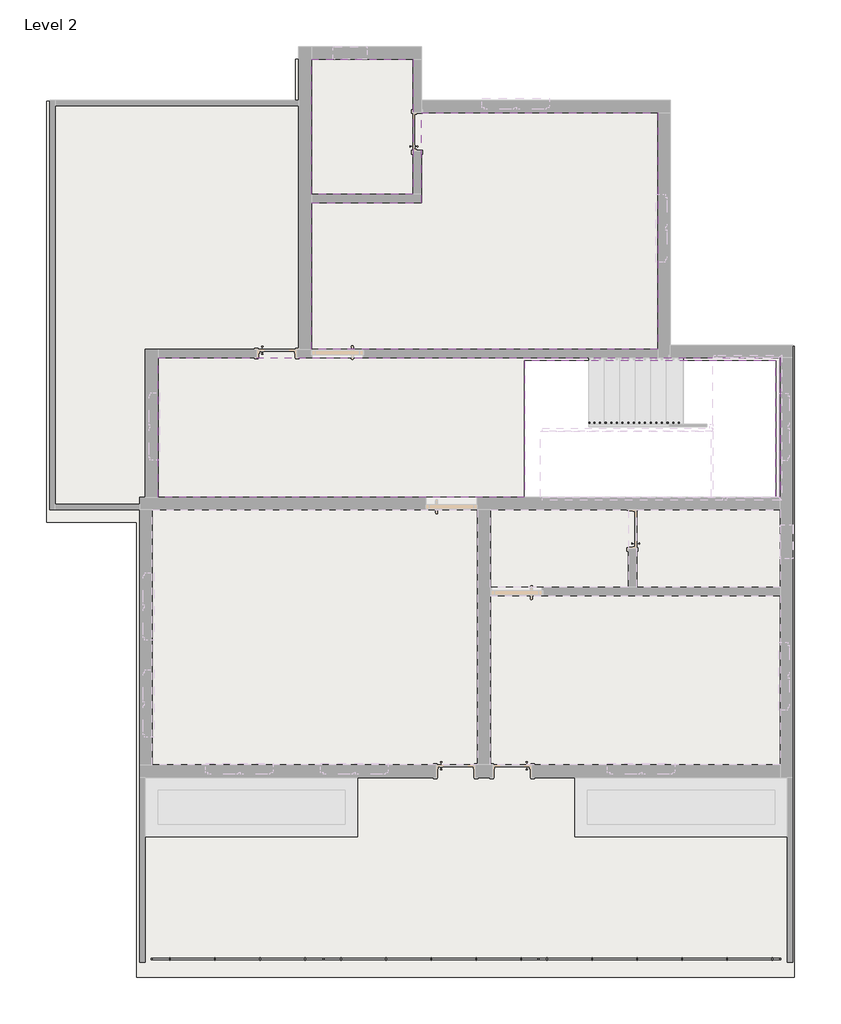
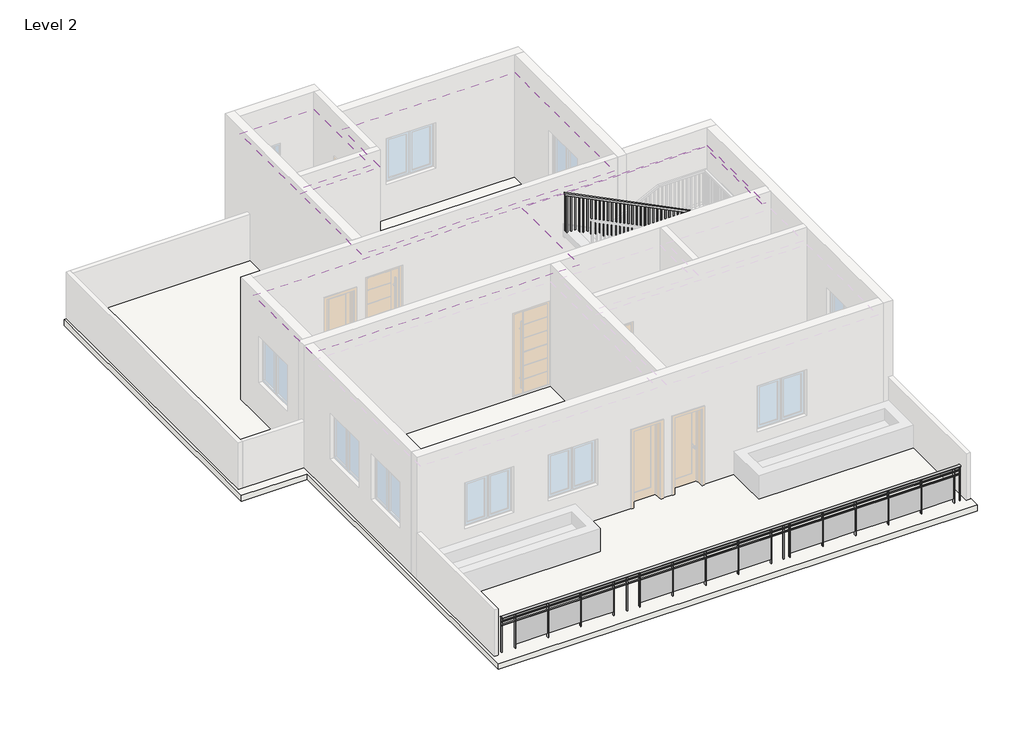
# One storey, part 2 of 3: 3 coverings, 2 railings, 1 slab.
"""IFC4 building model written with IfcOpenShell, lengths in millimetres."""

from ifc_helpers import new_model, si_unit, point, frame, origin, place, context, project, spatial, polyline, ellipse_curve, trimmed, outline, extrude, faceted_brep, element, save
from ifc_brep_helpers import plane_surface, extruded_surface, advanced_brep

model = new_model("IFC4")

# Units and contexts
model_context = context("Model", 3, world=origin())
ifc_project = project(units=[si_unit("LENGTHUNIT", "METRE", prefix="MILLI")], contexts=[model_context])

# Site, building, storey
site = spatial("IfcSite", under=ifc_project)
building = spatial("IfcBuilding", under=site)
storey = spatial("IfcBuildingStorey", under=building, Name="Level 2", Elevation=3200.4)

# Coverings
placement = place(None, origin())
element("IfcCovering", 1, ObjectType="2' x 4' ACT System", at=placement, inside=storey, context=model_context, shape_type="SweptSolid", body=[
    extrude(outline(polyline([(-10924.6183666, 3536.1503619), (-17173.0183666, 3536.1503619), (-17173.0183666, 6177.7503619), (-15191.8183666, 6177.7503619), (-15191.8183666, 7803.3503619), (-10924.6183666, 7803.3503619), (-10924.6183666, 3536.1503619)])), frame((0.0, 0.0, 6248.4), z_axis=(0.0, 0.0, 1.0), x_axis=(1.0, 0.0, 0.0)), (0.0, 0.0, 1.0), 57.15),
])
element("IfcCovering", 2, ObjectType="2' x 4' ACT System", at=placement, inside=storey, context=model_context, shape_type="SweptSolid", body=[
    extrude(outline(polyline([(-19941.6183666, 3383.7503619), (-10810.3183666, 3383.7503619), (-8714.8183666, 3383.7503619), (-8714.8183666, 869.1503619), (-8791.0183666, 869.1503619), (-8791.0183666, 3332.9503619), (-13326.4629678, 3332.9503619), (-13326.4629678, 869.1503619), (-19941.6183666, 869.1503619), (-19941.6183666, 3383.7503619)])), frame((0.0, 0.0, 6248.4), z_axis=(0.0, 0.0, 1.0), x_axis=(1.0, 0.0, 0.0)), (0.0, 0.0, 1.0), 57.15),
])
element("IfcCovering", 3, ObjectType="2' x 4' ACT System", at=placement, inside=storey, context=model_context, shape_type="SweptSolid", body=[
    extrude(outline(polyline([(-15344.2183666, 6330.1503619), (-17173.0183666, 6330.1503619), (-17173.0183666, 8768.5503619), (-15344.2183666, 8768.5503619), (-15344.2183666, 6330.1503619)])), frame((0.0, 0.0, 6248.4), z_axis=(0.0, 0.0, 1.0), x_axis=(1.0, 0.0, 0.0)), (0.0, 0.0, 1.0), 57.15),
])

# Railings
element("IfcRailing", 4, ObjectType="Glass Panel - Bottom Fill", at=placement, inside=storey, context=model_context, shape_type="SolidModel", body=[
    advanced_brep(
    [(-8708.4683666, -7493.7996381, 4419.6), (-8708.4683666, -7417.5996381, 4419.6), (-20062.2683666, -7493.7996381, 4419.6), (-20062.2683666, -7417.5996381, 4419.6)],
    [
        (0, 1, ellipse_curve(frame((-8708.4683666, -7455.6996381, 4419.6), z_axis=(1.0, 0.0, 0.0), x_axis=(0.0, 1.0, 0.0)), 38.1, 28.575)),
        (1, 0, ellipse_curve(frame((-8708.4683666, -7455.6996381, 4419.6), z_axis=(1.0, 0.0, 0.0), x_axis=(0.0, 1.0, 0.0)), 38.1, 28.575)),
        (2, 3, ellipse_curve(frame((-20062.2683666, -7455.6996381, 4419.6), z_axis=(-1.0, 0.0, 0.0), x_axis=(0.0, 1.0, 0.0)), 38.1, 28.575)),
        (3, 2, ellipse_curve(frame((-20062.2683666, -7455.6996381, 4419.6), z_axis=(-1.0, 0.0, 0.0), x_axis=(0.0, 1.0, 0.0)), 38.1, 28.575)),
        (0, 2),
        (3, 1),
    ],
    [
        plane_surface(frame((-8708.4683666, -7455.6996381, 4419.6), z_axis=(1.0, 0.0, 0.0), x_axis=(0.0, -1.0, 0.0))),
        plane_surface(frame((-20062.2683666, -7455.6996381, 4419.6), z_axis=(-1.0, 0.0, 0.0), x_axis=(0.0, -1.0, 0.0))),
        extruded_surface(trimmed(ellipse_curve(frame((-20062.2683666, -7455.6996381, 4419.6), z_axis=(1.0, 0.0, 0.0), x_axis=(0.0, 1.0, 0.0)), 38.1, 28.575), [point((-20062.2683666, -7493.7996381, 4419.6))], [point((-20062.2683666, -7417.5996381, 4419.6))], True, "CARTESIAN"), (11353.800000000001, 0.0, 0.0), 11353.800000000001),
        extruded_surface(trimmed(ellipse_curve(frame((-20062.2683666, -7455.6996381, 4419.6), z_axis=(1.0, 0.0, 0.0), x_axis=(0.0, 1.0, 0.0)), 38.1, 28.575), [point((-20062.2683666, -7417.5996381, 4419.6))], [point((-20062.2683666, -7493.7996381, 4419.6))], True, "CARTESIAN"), (11353.800000000001, 0.0, 0.0), 11353.800000000001),
    ],
    [
        (0, [[1, 2]]),
        (1, [[3, 4]]),
        (2, [[-1, 5, -4, 6]]),
        (3, [[-2, -6, -3, -5]]),
    ],
),
    extrude(outline(polyline([(-8708.4683666, -7442.9996381), (-8708.4683666, -7468.3996381), (-20062.2683666, -7468.3996381), (-20062.2683666, -7442.9996381), (-8708.4683666, -7442.9996381)])), frame((0.0, 0.0, 4305.3), z_axis=(0.0, 0.0, 1.0), x_axis=(1.0, 0.0, 0.0)), (0.0, 0.0, 1.0), 25.4),
    extrude(outline(polyline([(-8708.4683666, -7442.9996381), (-8708.4683666, -7468.3996381), (-20062.2683666, -7468.3996381), (-20062.2683666, -7442.9996381), (-8708.4683666, -7442.9996381)])), frame((0.0, 0.0, 4203.7), z_axis=(0.0, 0.0, 1.0), x_axis=(1.0, 0.0, 0.0)), (0.0, 0.0, 1.0), 25.4),
    extrude(outline(polyline([(-19719.9291774, -7430.2996381), (-19719.9291774, -7481.0996381), (-19732.6291774, -7481.0996381), (-19732.6291774, -7430.2996381), (-19719.9291774, -7430.2996381)])), frame((0.0, 0.0, 3505.2), z_axis=(0.0, 0.0, 1.0), x_axis=(1.0, 0.0, 0.0)), (0.0, 0.0, 1.0), 885.825),
    extrude(outline(polyline([(-18913.4791774, -7462.2347951), (-19726.2791774, -7462.2347951), (-19726.2791774, -7455.8847951), (-18913.4791774, -7455.8847951), (-18913.4791774, -7462.2347951)])), frame((0.0, 0.0, 3606.8), z_axis=(0.0, 0.0, 1.0), x_axis=(1.0, 0.0, 0.0)), (0.0, 0.0, 1.0), 596.9),
    extrude(outline(polyline([(-18907.1291774, -7430.2996381), (-18907.1291774, -7481.0996381), (-18919.8291774, -7481.0996381), (-18919.8291774, -7430.2996381), (-18907.1291774, -7430.2996381)])), frame((0.0, 0.0, 3505.2), z_axis=(0.0, 0.0, 1.0), x_axis=(1.0, 0.0, 0.0)), (0.0, 0.0, 1.0), 885.825),
    extrude(outline(polyline([(-18100.6791774, -7462.2347951), (-18913.4791774, -7462.2347951), (-18913.4791774, -7455.8847951), (-18100.6791774, -7455.8847951), (-18100.6791774, -7462.2347951)])), frame((0.0, 0.0, 3606.8), z_axis=(0.0, 0.0, 1.0), x_axis=(1.0, 0.0, 0.0)), (0.0, 0.0, 1.0), 596.9),
    extrude(outline(polyline([(-18094.3291774, -7430.2996381), (-18094.3291774, -7481.0996381), (-18107.0291774, -7481.0996381), (-18107.0291774, -7430.2996381), (-18094.3291774, -7430.2996381)])), frame((0.0, 0.0, 3505.2), z_axis=(0.0, 0.0, 1.0), x_axis=(1.0, 0.0, 0.0)), (0.0, 0.0, 1.0), 885.825),
    extrude(outline(polyline([(-17287.8791774, -7462.2347951), (-18100.6791774, -7462.2347951), (-18100.6791774, -7455.8847951), (-17287.8791774, -7455.8847951), (-17287.8791774, -7462.2347951)])), frame((0.0, 0.0, 3606.8), z_axis=(0.0, 0.0, 1.0), x_axis=(1.0, 0.0, 0.0)), (0.0, 0.0, 1.0), 596.9),
    extrude(outline(polyline([(-17281.5291774, -7430.2996381), (-17281.5291774, -7481.0996381), (-17294.2291774, -7481.0996381), (-17294.2291774, -7430.2996381), (-17281.5291774, -7430.2996381)])), frame((0.0, 0.0, 3505.2), z_axis=(0.0, 0.0, 1.0), x_axis=(1.0, 0.0, 0.0)), (0.0, 0.0, 1.0), 885.825),
    extrude(outline(polyline([(-16632.6150671, -7430.2996381), (-16632.6150671, -7481.0996381), (-16645.3150671, -7481.0996381), (-16645.3150671, -7430.2996381), (-16632.6150671, -7430.2996381)])), frame((0.0, 0.0, 3505.2), z_axis=(0.0, 0.0, 1.0), x_axis=(1.0, 0.0, 0.0)), (0.0, 0.0, 1.0), 885.825),
    extrude(outline(polyline([(-15826.1650671, -7462.2347951), (-16638.9650671, -7462.2347951), (-16638.9650671, -7455.8847951), (-15826.1650671, -7455.8847951), (-15826.1650671, -7462.2347951)])), frame((0.0, 0.0, 3606.8), z_axis=(0.0, 0.0, 1.0), x_axis=(1.0, 0.0, 0.0)), (0.0, 0.0, 1.0), 596.9),
    extrude(outline(polyline([(-15819.8150671, -7430.2996381), (-15819.8150671, -7481.0996381), (-15832.5150671, -7481.0996381), (-15832.5150671, -7430.2996381), (-15819.8150671, -7430.2996381)])), frame((0.0, 0.0, 3505.2), z_axis=(0.0, 0.0, 1.0), x_axis=(1.0, 0.0, 0.0)), (0.0, 0.0, 1.0), 885.825),
    extrude(outline(polyline([(-15013.3650671, -7462.2347951), (-15826.1650671, -7462.2347951), (-15826.1650671, -7455.8847951), (-15013.3650671, -7455.8847951), (-15013.3650671, -7462.2347951)])), frame((0.0, 0.0, 3606.8), z_axis=(0.0, 0.0, 1.0), x_axis=(1.0, 0.0, 0.0)), (0.0, 0.0, 1.0), 596.9),
    extrude(outline(polyline([(-15007.0150671, -7430.2996381), (-15007.0150671, -7481.0996381), (-15019.7150671, -7481.0996381), (-15019.7150671, -7430.2996381), (-15007.0150671, -7430.2996381)])), frame((0.0, 0.0, 3505.2), z_axis=(0.0, 0.0, 1.0), x_axis=(1.0, 0.0, 0.0)), (0.0, 0.0, 1.0), 885.825),
    extrude(outline(polyline([(-14200.5650671, -7462.2347951), (-15013.3650671, -7462.2347951), (-15013.3650671, -7455.8847951), (-14200.5650671, -7455.8847951), (-14200.5650671, -7462.2347951)])), frame((0.0, 0.0, 3606.8), z_axis=(0.0, 0.0, 1.0), x_axis=(1.0, 0.0, 0.0)), (0.0, 0.0, 1.0), 596.9),
    extrude(outline(polyline([(-14194.2150671, -7430.2996381), (-14194.2150671, -7481.0996381), (-14206.9150671, -7481.0996381), (-14206.9150671, -7430.2996381), (-14194.2150671, -7430.2996381)])), frame((0.0, 0.0, 3505.2), z_axis=(0.0, 0.0, 1.0), x_axis=(1.0, 0.0, 0.0)), (0.0, 0.0, 1.0), 885.825),
    extrude(outline(polyline([(-13387.7650671, -7462.2347951), (-14200.5650671, -7462.2347951), (-14200.5650671, -7455.8847951), (-13387.7650671, -7455.8847951), (-13387.7650671, -7462.2347951)])), frame((0.0, 0.0, 3606.8), z_axis=(0.0, 0.0, 1.0), x_axis=(1.0, 0.0, 0.0)), (0.0, 0.0, 1.0), 596.9),
    extrude(outline(polyline([(-13381.4150671, -7430.2996381), (-13381.4150671, -7481.0996381), (-13394.1150671, -7481.0996381), (-13394.1150671, -7430.2996381), (-13381.4150671, -7430.2996381)])), frame((0.0, 0.0, 3505.2), z_axis=(0.0, 0.0, 1.0), x_axis=(1.0, 0.0, 0.0)), (0.0, 0.0, 1.0), 885.825),
    extrude(outline(polyline([(-12917.3042563, -7430.2996381), (-12917.3042563, -7481.0996381), (-12930.0042563, -7481.0996381), (-12930.0042563, -7430.2996381), (-12917.3042563, -7430.2996381)])), frame((0.0, 0.0, 3505.2), z_axis=(0.0, 0.0, 1.0), x_axis=(1.0, 0.0, 0.0)), (0.0, 0.0, 1.0), 885.825),
    extrude(outline(polyline([(-12110.8542563, -7462.2347951), (-12923.6542563, -7462.2347951), (-12923.6542563, -7455.8847951), (-12110.8542563, -7455.8847951), (-12110.8542563, -7462.2347951)])), frame((0.0, 0.0, 3606.8), z_axis=(0.0, 0.0, 1.0), x_axis=(1.0, 0.0, 0.0)), (0.0, 0.0, 1.0), 596.9),
    extrude(outline(polyline([(-12104.5042563, -7430.2996381), (-12104.5042563, -7481.0996381), (-12117.2042563, -7481.0996381), (-12117.2042563, -7430.2996381), (-12104.5042563, -7430.2996381)])), frame((0.0, 0.0, 3505.2), z_axis=(0.0, 0.0, 1.0), x_axis=(1.0, 0.0, 0.0)), (0.0, 0.0, 1.0), 885.825),
    extrude(outline(polyline([(-11298.0542563, -7462.2347951), (-12110.8542563, -7462.2347951), (-12110.8542563, -7455.8847951), (-11298.0542563, -7455.8847951), (-11298.0542563, -7462.2347951)])), frame((0.0, 0.0, 3606.8), z_axis=(0.0, 0.0, 1.0), x_axis=(1.0, 0.0, 0.0)), (0.0, 0.0, 1.0), 596.9),
    extrude(outline(polyline([(-11291.7042563, -7430.2996381), (-11291.7042563, -7481.0996381), (-11304.4042563, -7481.0996381), (-11304.4042563, -7430.2996381), (-11291.7042563, -7430.2996381)])), frame((0.0, 0.0, 3505.2), z_axis=(0.0, 0.0, 1.0), x_axis=(1.0, 0.0, 0.0)), (0.0, 0.0, 1.0), 885.825),
    extrude(outline(polyline([(-10485.2542563, -7462.2347951), (-11298.0542563, -7462.2347951), (-11298.0542563, -7455.8847951), (-10485.2542563, -7455.8847951), (-10485.2542563, -7462.2347951)])), frame((0.0, 0.0, 3606.8), z_axis=(0.0, 0.0, 1.0), x_axis=(1.0, 0.0, 0.0)), (0.0, 0.0, 1.0), 596.9),
    extrude(outline(polyline([(-10478.9042563, -7430.2996381), (-10478.9042563, -7481.0996381), (-10491.6042563, -7481.0996381), (-10491.6042563, -7430.2996381), (-10478.9042563, -7430.2996381)])), frame((0.0, 0.0, 3505.2), z_axis=(0.0, 0.0, 1.0), x_axis=(1.0, 0.0, 0.0)), (0.0, 0.0, 1.0), 885.825),
    extrude(outline(polyline([(-9672.4542563, -7462.2347951), (-10485.2542563, -7462.2347951), (-10485.2542563, -7455.8847951), (-9672.4542563, -7455.8847951), (-9672.4542563, -7462.2347951)])), frame((0.0, 0.0, 3606.8), z_axis=(0.0, 0.0, 1.0), x_axis=(1.0, 0.0, 0.0)), (0.0, 0.0, 1.0), 596.9),
    extrude(outline(polyline([(-9666.1042563, -7430.2996381), (-9666.1042563, -7481.0996381), (-9678.8042563, -7481.0996381), (-9678.8042563, -7430.2996381), (-9666.1042563, -7430.2996381)])), frame((0.0, 0.0, 3505.2), z_axis=(0.0, 0.0, 1.0), x_axis=(1.0, 0.0, 0.0)), (0.0, 0.0, 1.0), 885.825),
    extrude(outline(polyline([(-8859.6542563, -7462.2347951), (-9672.4542563, -7462.2347951), (-9672.4542563, -7455.8847951), (-8859.6542563, -7455.8847951), (-8859.6542563, -7462.2347951)])), frame((0.0, 0.0, 3606.8), z_axis=(0.0, 0.0, 1.0), x_axis=(1.0, 0.0, 0.0)), (0.0, 0.0, 1.0), 596.9),
    extrude(outline(polyline([(-8853.3042563, -7430.2996381), (-8853.3042563, -7481.0996381), (-8866.0042563, -7481.0996381), (-8866.0042563, -7430.2996381), (-8853.3042563, -7430.2996381)])), frame((0.0, 0.0, 3505.2), z_axis=(0.0, 0.0, 1.0), x_axis=(1.0, 0.0, 0.0)), (0.0, 0.0, 1.0), 885.825),
    extrude(outline(polyline([(-16942.3649883, -7446.1746381), (-16942.3649883, -7465.2246381), (-16961.4149883, -7465.2246381), (-16961.4149883, -7446.1746381), (-16942.3649883, -7446.1746381)])), frame((0.0, 0.0, 3505.2), z_axis=(0.0, 0.0, 1.0), x_axis=(1.0, 0.0, 0.0)), (0.0, 0.0, 1.0), 885.825),
    extrude(outline(polyline([(-13065.3151459, -7446.1746381), (-13065.3151459, -7465.2246381), (-13084.3651459, -7465.2246381), (-13084.3651459, -7446.1746381), (-13065.3151459, -7446.1746381)])), frame((0.0, 0.0, 3505.2), z_axis=(0.0, 0.0, 1.0), x_axis=(1.0, 0.0, 0.0)), (0.0, 0.0, 1.0), 885.825),
    extrude(outline(polyline([(-20049.5683666, -7446.1746381), (-20049.5683666, -7465.2246381), (-20068.6183666, -7465.2246381), (-20068.6183666, -7446.1746381), (-20049.5683666, -7446.1746381)])), frame((0.0, 0.0, 3505.2), z_axis=(0.0, 0.0, 1.0), x_axis=(1.0, 0.0, 0.0)), (0.0, 0.0, 1.0), 885.825),
    extrude(outline(polyline([(-8702.1183666, -7446.1746381), (-8702.1183666, -7465.2246381), (-8721.1683666, -7465.2246381), (-8721.1683666, -7446.1746381), (-8702.1183666, -7446.1746381)])), frame((0.0, 0.0, 3505.2), z_axis=(0.0, 0.0, 1.0), x_axis=(1.0, 0.0, 0.0)), (0.0, 0.0, 1.0), 885.825),
])
element("IfcRailing", 5, ObjectType="Handrail - Rectangular", at=placement, inside=storey, context=model_context, shape_type="SolidModel", body=[
    faceted_brep([(-12169.2183666, 2240.7503619, 4532.2434783), (-12169.2183666, 2240.7503619, 4475.4921787), (-12169.2183666, 2189.9503619, 4475.4921787), (-12169.2183666, 2189.9503619, 4532.2434783), (-10010.2183666, 2240.7503619, 5607.4766798), (-9959.4183666, 2240.7503619, 5576.024985), (-9959.4183666, 2189.9503619, 5576.024985), (-10010.2183666, 2189.9503619, 5607.4766798), (-10010.2183666, 2240.7503619, 5645.426087), (-9959.4183666, 2240.7503619, 5594.626087), (-9959.4183666, 2189.9503619, 5594.626087), (-10010.2183666, 2189.9503619, 5645.426087), (-9883.2183666, 2240.7503619, 5645.426087), (-9883.2183666, 2240.7503619, 5594.626087), (-9934.0183666, 2189.9503619, 5594.626087), (-9934.0183666, 2189.9503619, 5645.426087), (-9883.2183666, 2113.7503619, 5645.426087), (-9883.2183666, 2113.7503619, 5594.626087), (-9934.0183666, 2113.7503619, 5594.626087), (-9934.0183666, 2113.7503619, 5645.426087), (-9883.2183666, 2062.9503619, 5645.426087), (-9934.0183666, 2062.9503619, 5645.426087), (-9934.0183666, 2012.1503619, 5594.626087), (-9883.2183666, 2012.1503619, 5594.626087)], [[[0, 1, 2, 3]], [[1, 0, 4, 5]], [[2, 1, 5, 6]], [[3, 2, 6, 7]], [[0, 3, 7, 4]], [[5, 4, 8, 9]], [[6, 5, 9, 10]], [[7, 6, 10, 11]], [[4, 7, 11, 8]], [[9, 8, 12, 13]], [[10, 9, 13, 14]], [[11, 10, 14, 15]], [[8, 11, 15, 12]], [[13, 12, 16, 17]], [[14, 13, 17, 18]], [[15, 14, 18, 19]], [[12, 15, 19, 16]], [[20, 21, 22, 23]], [[17, 16, 20, 23]], [[18, 17, 23, 22]], [[19, 18, 22, 21]], [[16, 19, 21, 20]]]),
    faceted_brep([(-9883.2183666, 2062.9503619, 5645.426087), (-9883.2183666, 2012.1503619, 5594.626087), (-9934.0183666, 2012.1503619, 5594.626087), (-9934.0183666, 2062.9503619, 5645.426087), (-9883.2183666, 2062.9503619, 5759.2743083), (-9934.0183666, 2062.9503619, 5727.8226135), (-9934.0183666, 2012.1503619, 5727.8226135), (-9883.2183666, 2012.1503619, 5759.2743083)], [[[0, 1, 2, 3]], [[4, 5, 6, 7]], [[1, 0, 4, 7]], [[2, 1, 7, 6]], [[3, 2, 6, 5]], [[0, 3, 5, 4]]]),
    faceted_brep([(-9883.2183666, 2012.1503619, 5759.2743083), (-9934.0183666, 2012.1503619, 5727.8226135), (-9934.0183666, 2062.9503619, 5727.8226135), (-9883.2183666, 2062.9503619, 5759.2743083), (-13007.4183666, 2012.1503619, 7315.2), (-13007.4183666, 2062.9503619, 7315.2), (-13007.4183666, 2062.9503619, 7258.4487005), (-13007.4183666, 2012.1503619, 7258.4487005)], [[[0, 1, 2, 3]], [[4, 5, 6, 7]], [[1, 0, 4, 7]], [[2, 1, 7, 6]], [[3, 2, 6, 5]], [[0, 3, 5, 4]]]),
    extrude(outline(polyline([(7228.4054198, -12947.0933666), (7237.8927716, -12966.1433666), (6261.6521739, -12966.1433666), (6261.6521739, -12947.0933666), (7228.4054198, -12947.0933666)])), frame((0.0, 2028.0253619, 0.0), z_axis=(0.0, 1.0, 0.0), x_axis=(0.0, 0.0, 1.0)), (0.0, 0.0, 1.0), 19.05),
    extrude(outline(polyline([(7177.8062103, -12845.4933666), (7187.2935621, -12864.5433666), (6261.6521739, -12864.5433666), (6261.6521739, -12845.4933666), (7177.8062103, -12845.4933666)])), frame((0.0, 2028.0253619, 0.0), z_axis=(0.0, 1.0, 0.0), x_axis=(0.0, 0.0, 1.0)), (0.0, 0.0, 1.0), 19.05),
    extrude(outline(polyline([(7127.2070008, -12743.8933666), (7136.6943526, -12762.9433666), (6261.6521739, -12762.9433666), (6261.6521739, -12743.8933666), (7127.2070008, -12743.8933666)])), frame((0.0, 2028.0253619, 0.0), z_axis=(0.0, 1.0, 0.0), x_axis=(0.0, 0.0, 1.0)), (0.0, 0.0, 1.0), 19.05),
    extrude(outline(polyline([(7076.6077914, -12642.2933666), (7086.0951431, -12661.3433666), (6122.5043478, -12661.3433666), (6122.5043478, -12642.2933666), (7076.6077914, -12642.2933666)])), frame((0.0, 2028.0253619, 0.0), z_axis=(0.0, 1.0, 0.0), x_axis=(0.0, 0.0, 1.0)), (0.0, 0.0, 1.0), 19.05),
    extrude(outline(polyline([(7026.0085819, -12540.6933666), (7035.4959337, -12559.7433666), (6122.5043478, -12559.7433666), (6122.5043478, -12540.6933666), (7026.0085819, -12540.6933666)])), frame((0.0, 2028.0253619, 0.0), z_axis=(0.0, 1.0, 0.0), x_axis=(0.0, 0.0, 1.0)), (0.0, 0.0, 1.0), 19.05),
    extrude(outline(polyline([(6975.4093724, -12439.0933666), (6984.8967242, -12458.1433666), (6122.5043478, -12458.1433666), (6122.5043478, -12439.0933666), (6975.4093724, -12439.0933666)])), frame((0.0, 2028.0253619, 0.0), z_axis=(0.0, 1.0, 0.0), x_axis=(0.0, 0.0, 1.0)), (0.0, 0.0, 1.0), 19.05),
    extrude(outline(polyline([(6924.8101629, -12337.4933666), (6934.2975147, -12356.5433666), (5983.3565217, -12356.5433666), (5983.3565217, -12337.4933666), (6924.8101629, -12337.4933666)])), frame((0.0, 2028.0253619, 0.0), z_axis=(0.0, 1.0, 0.0), x_axis=(0.0, 0.0, 1.0)), (0.0, 0.0, 1.0), 19.05),
    extrude(outline(polyline([(6874.2109534, -12235.8933666), (6883.6983052, -12254.9433666), (5983.3565217, -12254.9433666), (5983.3565217, -12235.8933666), (6874.2109534, -12235.8933666)])), frame((0.0, 2028.0253619, 0.0), z_axis=(0.0, 1.0, 0.0), x_axis=(0.0, 0.0, 1.0)), (0.0, 0.0, 1.0), 19.05),
    extrude(outline(polyline([(6823.6117439, -12134.2933666), (6833.0990957, -12153.3433666), (5844.2086957, -12153.3433666), (5844.2086957, -12134.2933666), (6823.6117439, -12134.2933666)])), frame((0.0, 2028.0253619, 0.0), z_axis=(0.0, 1.0, 0.0), x_axis=(0.0, 0.0, 1.0)), (0.0, 0.0, 1.0), 19.05),
    extrude(outline(polyline([(6773.0125344, -12032.6933666), (6782.4998862, -12051.7433666), (5844.2086957, -12051.7433666), (5844.2086957, -12032.6933666), (6773.0125344, -12032.6933666)])), frame((0.0, 2028.0253619, 0.0), z_axis=(0.0, 1.0, 0.0), x_axis=(0.0, 0.0, 1.0)), (0.0, 0.0, 1.0), 19.05),
    extrude(outline(polyline([(6722.413325, -11931.0933666), (6731.9006767, -11950.1433666), (5844.2086957, -11950.1433666), (5844.2086957, -11931.0933666), (6722.413325, -11931.0933666)])), frame((0.0, 2028.0253619, 0.0), z_axis=(0.0, 1.0, 0.0), x_axis=(0.0, 0.0, 1.0)), (0.0, 0.0, 1.0), 19.05),
    extrude(outline(polyline([(6671.8141155, -11829.4933666), (6681.3014673, -11848.5433666), (5705.0608696, -11848.5433666), (5705.0608696, -11829.4933666), (6671.8141155, -11829.4933666)])), frame((0.0, 2028.0253619, 0.0), z_axis=(0.0, 1.0, 0.0), x_axis=(0.0, 0.0, 1.0)), (0.0, 0.0, 1.0), 19.05),
    extrude(outline(polyline([(6621.214906, -11727.8933666), (6630.7022578, -11746.9433666), (5705.0608696, -11746.9433666), (5705.0608696, -11727.8933666), (6621.214906, -11727.8933666)])), frame((0.0, 2028.0253619, 0.0), z_axis=(0.0, 1.0, 0.0), x_axis=(0.0, 0.0, 1.0)), (0.0, 0.0, 1.0), 19.05),
    extrude(outline(polyline([(6570.6156965, -11626.2933666), (6580.1030483, -11645.3433666), (5705.0608696, -11645.3433666), (5705.0608696, -11626.2933666), (6570.6156965, -11626.2933666)])), frame((0.0, 2028.0253619, 0.0), z_axis=(0.0, 1.0, 0.0), x_axis=(0.0, 0.0, 1.0)), (0.0, 0.0, 1.0), 19.05),
    extrude(outline(polyline([(6520.016487, -11524.6933666), (6529.5038388, -11543.7433666), (5565.9130435, -11543.7433666), (5565.9130435, -11524.6933666), (6520.016487, -11524.6933666)])), frame((0.0, 2028.0253619, 0.0), z_axis=(0.0, 1.0, 0.0), x_axis=(0.0, 0.0, 1.0)), (0.0, 0.0, 1.0), 19.05),
    extrude(outline(polyline([(6469.4172775, -11423.0933666), (6478.9046293, -11442.1433666), (5565.9130435, -11442.1433666), (5565.9130435, -11423.0933666), (6469.4172775, -11423.0933666)])), frame((0.0, 2028.0253619, 0.0), z_axis=(0.0, 1.0, 0.0), x_axis=(0.0, 0.0, 1.0)), (0.0, 0.0, 1.0), 19.05),
    extrude(outline(polyline([(6418.818068, -11321.4933666), (6428.3054198, -11340.5433666), (5565.9130435, -11340.5433666), (5565.9130435, -11321.4933666), (6418.818068, -11321.4933666)])), frame((0.0, 2028.0253619, 0.0), z_axis=(0.0, 1.0, 0.0), x_axis=(0.0, 0.0, 1.0)), (0.0, 0.0, 1.0), 19.05),
    extrude(outline(polyline([(6368.2188586, -11219.8933666), (6377.7062103, -11238.9433666), (5426.7652174, -11238.9433666), (5426.7652174, -11219.8933666), (6368.2188586, -11219.8933666)])), frame((0.0, 2028.0253619, 0.0), z_axis=(0.0, 1.0, 0.0), x_axis=(0.0, 0.0, 1.0)), (0.0, 0.0, 1.0), 19.05),
    extrude(outline(polyline([(6317.6196491, -11118.2933666), (6327.1070008, -11137.3433666), (5426.7652174, -11137.3433666), (5426.7652174, -11118.2933666), (6317.6196491, -11118.2933666)])), frame((0.0, 2028.0253619, 0.0), z_axis=(0.0, 1.0, 0.0), x_axis=(0.0, 0.0, 1.0)), (0.0, 0.0, 1.0), 19.05),
    extrude(outline(polyline([(6267.0204396, -11016.6933666), (6276.5077914, -11035.7433666), (5287.6173913, -11035.7433666), (5287.6173913, -11016.6933666), (6267.0204396, -11016.6933666)])), frame((0.0, 2028.0253619, 0.0), z_axis=(0.0, 1.0, 0.0), x_axis=(0.0, 0.0, 1.0)), (0.0, 0.0, 1.0), 19.05),
    extrude(outline(polyline([(6216.4212301, -10915.0933666), (6225.9085819, -10934.1433666), (5287.6173913, -10934.1433666), (5287.6173913, -10915.0933666), (6216.4212301, -10915.0933666)])), frame((0.0, 2028.0253619, 0.0), z_axis=(0.0, 1.0, 0.0), x_axis=(0.0, 0.0, 1.0)), (0.0, 0.0, 1.0), 19.05),
    extrude(outline(polyline([(6165.8220206, -10813.4933666), (6175.3093724, -10832.5433666), (5287.6173913, -10832.5433666), (5287.6173913, -10813.4933666), (6165.8220206, -10813.4933666)])), frame((0.0, 2028.0253619, 0.0), z_axis=(0.0, 1.0, 0.0), x_axis=(0.0, 0.0, 1.0)), (0.0, 0.0, 1.0), 19.05),
    extrude(outline(polyline([(6115.2228111, -10711.8933666), (6124.7101629, -10730.9433666), (5148.4695652, -10730.9433666), (5148.4695652, -10711.8933666), (6115.2228111, -10711.8933666)])), frame((0.0, 2028.0253619, 0.0), z_axis=(0.0, 1.0, 0.0), x_axis=(0.0, 0.0, 1.0)), (0.0, 0.0, 1.0), 19.05),
    extrude(outline(polyline([(6064.6236016, -10610.2933666), (6074.1109534, -10629.3433666), (5148.4695652, -10629.3433666), (5148.4695652, -10610.2933666), (6064.6236016, -10610.2933666)])), frame((0.0, 2028.0253619, 0.0), z_axis=(0.0, 1.0, 0.0), x_axis=(0.0, 0.0, 1.0)), (0.0, 0.0, 1.0), 19.05),
    extrude(outline(polyline([(6014.0243922, -10508.6933666), (6023.5117439, -10527.7433666), (5148.4695652, -10527.7433666), (5148.4695652, -10508.6933666), (6014.0243922, -10508.6933666)])), frame((0.0, 2028.0253619, 0.0), z_axis=(0.0, 1.0, 0.0), x_axis=(0.0, 0.0, 1.0)), (0.0, 0.0, 1.0), 19.05),
    extrude(outline(polyline([(5963.4251827, -10407.0933666), (5972.9125344, -10426.1433666), (5009.3217391, -10426.1433666), (5009.3217391, -10407.0933666), (5963.4251827, -10407.0933666)])), frame((0.0, 2028.0253619, 0.0), z_axis=(0.0, 1.0, 0.0), x_axis=(0.0, 0.0, 1.0)), (0.0, 0.0, 1.0), 19.05),
    extrude(outline(polyline([(5912.8259732, -10305.4933666), (5922.313325, -10324.5433666), (5009.3217391, -10324.5433666), (5009.3217391, -10305.4933666), (5912.8259732, -10305.4933666)])), frame((0.0, 2028.0253619, 0.0), z_axis=(0.0, 1.0, 0.0), x_axis=(0.0, 0.0, 1.0)), (0.0, 0.0, 1.0), 19.05),
    extrude(outline(polyline([(5862.2267637, -10203.8933666), (5871.7141155, -10222.9433666), (5009.3217391, -10222.9433666), (5009.3217391, -10203.8933666), (5862.2267637, -10203.8933666)])), frame((0.0, 2028.0253619, 0.0), z_axis=(0.0, 1.0, 0.0), x_axis=(0.0, 0.0, 1.0)), (0.0, 0.0, 1.0), 19.05),
    extrude(outline(polyline([(5811.6275542, -10102.2933666), (5821.114906, -10121.3433666), (4870.173913, -10121.3433666), (4870.173913, -10102.2933666), (5811.6275542, -10102.2933666)])), frame((0.0, 2028.0253619, 0.0), z_axis=(0.0, 1.0, 0.0), x_axis=(0.0, 0.0, 1.0)), (0.0, 0.0, 1.0), 19.05),
    extrude(outline(polyline([(5761.0283447, -10000.6933666), (5770.5156965, -10019.7433666), (4870.173913, -10019.7433666), (4870.173913, -10000.6933666), (5761.0283447, -10000.6933666)])), frame((0.0, 2028.0253619, 0.0), z_axis=(0.0, 1.0, 0.0), x_axis=(0.0, 0.0, 1.0)), (0.0, 0.0, 1.0), 19.05),
    extrude(outline(polyline([(-9918.1433666, 2123.2753619), (-9899.0933666, 2123.2753619), (-9899.0933666, 2104.2253619), (-9918.1433666, 2104.2253619), (-9918.1433666, 2123.2753619)])), frame((0.0, 0.0, 4731.026087), z_axis=(0.0, 0.0, 1.0), x_axis=(1.0, 0.0, 0.0)), (0.0, 0.0, 1.0), 863.6),
    extrude(outline(polyline([(-9943.5433666, 2205.8253619), (-9943.5433666, 2224.8753619), (-9924.4933666, 2224.8753619), (-9924.4933666, 2205.8253619), (-9943.5433666, 2205.8253619)])), frame((0.0, 0.0, 4731.026087), z_axis=(0.0, 0.0, 1.0), x_axis=(1.0, 0.0, 0.0)), (0.0, 0.0, 1.0), 863.6),
    extrude(outline(polyline([(5542.8192538, -10026.0933666), (5533.331902, -10045.1433666), (4591.8782609, -10045.1433666), (4591.8782609, -10026.0933666), (5542.8192538, -10026.0933666)])), frame((0.0, 2205.8253619, 0.0), z_axis=(0.0, 1.0, 0.0), x_axis=(0.0, 0.0, 1.0)), (0.0, 0.0, 1.0), 19.05),
    extrude(outline(polyline([(5492.2200443, -10127.6933666), (5482.7326925, -10146.7433666), (4591.8782609, -10146.7433666), (4591.8782609, -10127.6933666), (5492.2200443, -10127.6933666)])), frame((0.0, 2205.8253619, 0.0), z_axis=(0.0, 1.0, 0.0), x_axis=(0.0, 0.0, 1.0)), (0.0, 0.0, 1.0), 19.05),
    extrude(outline(polyline([(5441.6208348, -10229.2933666), (5432.1334831, -10248.3433666), (4452.7304348, -10248.3433666), (4452.7304348, -10229.2933666), (5441.6208348, -10229.2933666)])), frame((0.0, 2205.8253619, 0.0), z_axis=(0.0, 1.0, 0.0), x_axis=(0.0, 0.0, 1.0)), (0.0, 0.0, 1.0), 19.05),
    extrude(outline(polyline([(5391.0216254, -10330.8933666), (5381.5342736, -10349.9433666), (4452.7304348, -10349.9433666), (4452.7304348, -10330.8933666), (5391.0216254, -10330.8933666)])), frame((0.0, 2205.8253619, 0.0), z_axis=(0.0, 1.0, 0.0), x_axis=(0.0, 0.0, 1.0)), (0.0, 0.0, 1.0), 19.05),
    extrude(outline(polyline([(5340.4224159, -10432.4933666), (5330.9350641, -10451.5433666), (4452.7304348, -10451.5433666), (4452.7304348, -10432.4933666), (5340.4224159, -10432.4933666)])), frame((0.0, 2205.8253619, 0.0), z_axis=(0.0, 1.0, 0.0), x_axis=(0.0, 0.0, 1.0)), (0.0, 0.0, 1.0), 19.05),
    extrude(outline(polyline([(5289.8232064, -10534.0933666), (5280.3358546, -10553.1433666), (4313.5826087, -10553.1433666), (4313.5826087, -10534.0933666), (5289.8232064, -10534.0933666)])), frame((0.0, 2205.8253619, 0.0), z_axis=(0.0, 1.0, 0.0), x_axis=(0.0, 0.0, 1.0)), (0.0, 0.0, 1.0), 19.05),
    extrude(outline(polyline([(5239.2239969, -10635.6933666), (5229.7366451, -10654.7433666), (4313.5826087, -10654.7433666), (4313.5826087, -10635.6933666), (5239.2239969, -10635.6933666)])), frame((0.0, 2205.8253619, 0.0), z_axis=(0.0, 1.0, 0.0), x_axis=(0.0, 0.0, 1.0)), (0.0, 0.0, 1.0), 19.05),
    extrude(outline(polyline([(5188.6247874, -10737.2933666), (5179.1374356, -10756.3433666), (4313.5826087, -10756.3433666), (4313.5826087, -10737.2933666), (5188.6247874, -10737.2933666)])), frame((0.0, 2205.8253619, 0.0), z_axis=(0.0, 1.0, 0.0), x_axis=(0.0, 0.0, 1.0)), (0.0, 0.0, 1.0), 19.05),
    extrude(outline(polyline([(5138.0255779, -10838.8933666), (5128.5382261, -10857.9433666), (4174.4347826, -10857.9433666), (4174.4347826, -10838.8933666), (5138.0255779, -10838.8933666)])), frame((0.0, 2205.8253619, 0.0), z_axis=(0.0, 1.0, 0.0), x_axis=(0.0, 0.0, 1.0)), (0.0, 0.0, 1.0), 19.05),
    extrude(outline(polyline([(5087.4263684, -10940.4933666), (5077.9390167, -10959.5433666), (4174.4347826, -10959.5433666), (4174.4347826, -10940.4933666), (5087.4263684, -10940.4933666)])), frame((0.0, 2205.8253619, 0.0), z_axis=(0.0, 1.0, 0.0), x_axis=(0.0, 0.0, 1.0)), (0.0, 0.0, 1.0), 19.05),
    extrude(outline(polyline([(5036.827159, -11042.0933666), (5027.3398072, -11061.1433666), (4174.4347826, -11061.1433666), (4174.4347826, -11042.0933666), (5036.827159, -11042.0933666)])), frame((0.0, 2205.8253619, 0.0), z_axis=(0.0, 1.0, 0.0), x_axis=(0.0, 0.0, 1.0)), (0.0, 0.0, 1.0), 19.05),
    extrude(outline(polyline([(4986.2279495, -11143.6933666), (4976.7405977, -11162.7433666), (4035.2869565, -11162.7433666), (4035.2869565, -11143.6933666), (4986.2279495, -11143.6933666)])), frame((0.0, 2205.8253619, 0.0), z_axis=(0.0, 1.0, 0.0), x_axis=(0.0, 0.0, 1.0)), (0.0, 0.0, 1.0), 19.05),
    extrude(outline(polyline([(4935.62874, -11245.2933666), (4926.1413882, -11264.3433666), (4035.2869565, -11264.3433666), (4035.2869565, -11245.2933666), (4935.62874, -11245.2933666)])), frame((0.0, 2205.8253619, 0.0), z_axis=(0.0, 1.0, 0.0), x_axis=(0.0, 0.0, 1.0)), (0.0, 0.0, 1.0), 19.05),
    extrude(outline(polyline([(4885.0295305, -11346.8933666), (4875.5421787, -11365.9433666), (3896.1391304, -11365.9433666), (3896.1391304, -11346.8933666), (4885.0295305, -11346.8933666)])), frame((0.0, 2205.8253619, 0.0), z_axis=(0.0, 1.0, 0.0), x_axis=(0.0, 0.0, 1.0)), (0.0, 0.0, 1.0), 19.05),
    extrude(outline(polyline([(4834.430321, -11448.4933666), (4824.9429692, -11467.5433666), (3896.1391304, -11467.5433666), (3896.1391304, -11448.4933666), (4834.430321, -11448.4933666)])), frame((0.0, 2205.8253619, 0.0), z_axis=(0.0, 1.0, 0.0), x_axis=(0.0, 0.0, 1.0)), (0.0, 0.0, 1.0), 19.05),
    extrude(outline(polyline([(4783.8311115, -11550.0933666), (4774.3437597, -11569.1433666), (3896.1391304, -11569.1433666), (3896.1391304, -11550.0933666), (4783.8311115, -11550.0933666)])), frame((0.0, 2205.8253619, 0.0), z_axis=(0.0, 1.0, 0.0), x_axis=(0.0, 0.0, 1.0)), (0.0, 0.0, 1.0), 19.05),
    extrude(outline(polyline([(4733.231902, -11651.6933666), (4723.7445503, -11670.7433666), (3756.9913043, -11670.7433666), (3756.9913043, -11651.6933666), (4733.231902, -11651.6933666)])), frame((0.0, 2205.8253619, 0.0), z_axis=(0.0, 1.0, 0.0), x_axis=(0.0, 0.0, 1.0)), (0.0, 0.0, 1.0), 19.05),
    extrude(outline(polyline([(4682.6326925, -11753.2933666), (4673.1453408, -11772.3433666), (3756.9913043, -11772.3433666), (3756.9913043, -11753.2933666), (4682.6326925, -11753.2933666)])), frame((0.0, 2205.8253619, 0.0), z_axis=(0.0, 1.0, 0.0), x_axis=(0.0, 0.0, 1.0)), (0.0, 0.0, 1.0), 19.05),
    extrude(outline(polyline([(4632.0334831, -11854.8933666), (4622.5461313, -11873.9433666), (3756.9913043, -11873.9433666), (3756.9913043, -11854.8933666), (4632.0334831, -11854.8933666)])), frame((0.0, 2205.8253619, 0.0), z_axis=(0.0, 1.0, 0.0), x_axis=(0.0, 0.0, 1.0)), (0.0, 0.0, 1.0), 19.05),
    extrude(outline(polyline([(4581.4342736, -11956.4933666), (4571.9469218, -11975.5433666), (3617.8434783, -11975.5433666), (3617.8434783, -11956.4933666), (4581.4342736, -11956.4933666)])), frame((0.0, 2205.8253619, 0.0), z_axis=(0.0, 1.0, 0.0), x_axis=(0.0, 0.0, 1.0)), (0.0, 0.0, 1.0), 19.05),
    extrude(outline(polyline([(4530.8350641, -12058.0933666), (4521.3477123, -12077.1433666), (3617.8434783, -12077.1433666), (3617.8434783, -12058.0933666), (4530.8350641, -12058.0933666)])), frame((0.0, 2205.8253619, 0.0), z_axis=(0.0, 1.0, 0.0), x_axis=(0.0, 0.0, 1.0)), (0.0, 0.0, 1.0), 19.05),
    extrude(outline(polyline([(-9918.1433666, 2047.0753619), (-9899.0933666, 2047.0753619), (-9899.0933666, 2028.0253619), (-9918.1433666, 2028.0253619), (-9918.1433666, 2047.0753619)])), frame((0.0, 0.0, 4731.026087), z_axis=(0.0, 0.0, 1.0), x_axis=(1.0, 0.0, 0.0)), (0.0, 0.0, 1.0), 863.6),
    extrude(outline(polyline([(-9918.1433666, 2205.8253619), (-9918.1433666, 2224.8753619), (-9899.0933666, 2224.8753619), (-9899.0933666, 2205.8253619), (-9918.1433666, 2205.8253619)])), frame((0.0, 0.0, 4731.026087), z_axis=(0.0, 0.0, 1.0), x_axis=(1.0, 0.0, 0.0)), (0.0, 0.0, 1.0), 863.6),
    extrude(outline(polyline([(7248.9613487, -12988.3683666), (7258.4487005, -13007.4183666), (6261.6521739, -13007.4183666), (6261.6521739, -12988.3683666), (7248.9613487, -12988.3683666)])), frame((0.0, 2028.0253619, 0.0), z_axis=(0.0, 1.0, 0.0), x_axis=(0.0, 0.0, 1.0)), (0.0, 0.0, 1.0), 19.05),
    extrude(outline(polyline([(4484.9795305, -12150.1683666), (4475.4921787, -12169.2183666), (3617.8434783, -12169.2183666), (3617.8434783, -12150.1683666), (4484.9795305, -12150.1683666)])), frame((0.0, 2205.8253619, 0.0), z_axis=(0.0, 1.0, 0.0), x_axis=(0.0, 0.0, 1.0)), (0.0, 0.0, 1.0), 19.05),
])

# Slab
element("IfcSlab", 6, ObjectType="Generic - 6\"", at=placement, inside=storey, context=model_context, shape_type="SweptSolid", body=[
    extrude(outline(polyline([(-20327.5006279, -7788.7606438), (-20327.5006279, 415.4393562), (-21953.1006279, 415.4393562), (-21953.1006279, 8010.0393562), (-17458.2535712, 8010.0393562), (-17458.2535712, 8772.0393562), (-15323.7006279, 8772.0393562), (-15323.7006279, 8010.0393562), (-10802.5006279, 8010.0393562), (-10802.5006279, 3590.4393562), (-8465.7006279, 3590.4393562), (-8465.7006279, -4181.9606438), (-8465.7006279, -7788.7606438), (-20327.5006279, -7788.7606438)]), holes=[polyline([(-13326.4629678, 3332.9503619), (-13326.4629678, 640.5503619), (-8791.0183666, 640.5503619), (-8791.0183666, 3332.9503619), (-13326.4629678, 3332.9503619)])]), frame((0.0, 0.0, 3352.8), z_axis=(0.0, 0.0, 1.0), x_axis=(1.0, 0.0, 0.0)), (0.0, 0.0, 1.0), 152.4),
])

save(model, "model.ifc")

# Revit data of these elements
# Type "2' x 4' ACT System"
#   Assembly Code = "C3030210"
#   built-in parameter 1002203 = 1 (stored number, unit not read)
#   built-in parameter 1002202 = 1 (stored number, unit not read)
#   Layers, outside or top first: 0' - 1 5/8" "Default" (function 1); 0' - 0 5/8" "Acoustic Ceiling Tile 24 x 48" (function 5)
# Type "Glass Panel - Bottom Fill"
#   Assembly Code = "C2010400"
#   built-in parameter 1008612 = 0.0416667 (stored number, unit not read)
#   built-in parameter 1008611 = 0.0416667 (stored number, unit not read)
#   built-in parameter 1008609 = 0.333333 (stored number, unit not read)
#   built-in parameter 1008604 = 0.166667 (stored number, unit not read)
#   built-in parameter 1008603 = 0.166667 (stored number, unit not read)
#   Railing Height = 3' - 0"
#   built-in parameter 1008630 = 2
#   built-in parameter 1008610 = 2
#   built-in parameter 1008618 = Baluster - Square : 3/4"
# Type "Handrail - Rectangular"
#   Assembly Code = "C2010400"
#   built-in parameter 1008612 = 0.0416667 (stored number, unit not read)
#   built-in parameter 1008611 = 0.0416667 (stored number, unit not read)
#   built-in parameter 1008609 = 0.333333 (stored number, unit not read)
#   built-in parameter 1008604 = 0.166667 (stored number, unit not read)
#   built-in parameter 1008603 = 0.166667 (stored number, unit not read)
#   Railing Height = 3' - 0"
#   built-in parameter 1008630 = 2
#   built-in parameter 1008610 = 2
#   built-in parameter 1008618 = Baluster - Square : 3/4"
# Type "Generic - 6\""
#   Assembly Code = "B1010"
#   Function = 0
#   Layers, outside or top first: 0' - 6" no material (function 1)
# Elements 1, 2, 3 (IfcCovering, "2' x 4' ACT System")
#   Height Offset From Level = 10' - 0"
#   Phase Created = New Construction
#   Materials on its faces: "Acoustic Ceiling Tile 24 x 48", "Default"
# Element 4 (IfcRailing, "Glass Panel - Bottom Fill")
#   built-in parameter 1008621 = 1 (stored number, unit not read)
#   Phase Created = New Construction
#   Materials on its faces: "Glass"
# Element 5 (IfcRailing, "Handrail - Rectangular")
#   Phase Created = New Construction
# Element 6 (IfcSlab, "Generic - 6\"")
#   built-in parameter 1001955 = 3.14159 (stored number, unit not read)
#   Height Offset From Level = 1' - 0"
#   Phase Created = New Construction
#   Materials on its faces: "9", "Default Floor", "Oak Flooring"
# Materials
#   "Default": colour RGB 127 127 127, transparency 0, Cost = 0
#   "Acoustic Ceiling Tile 24 x 48": class "Generic", colour RGB 229 229 229, transparency 0, Description = "Acoustic Ceiling Tile 24 x 48", Cost = 0
#   "Glass": class "Glass", colour RGB 0 128 192, transparency 0.75, Description = "Soda Lime Glass", Cost = 0
#   "9": class "Generic", colour RGB 120 120 120, transparency 0, Cost = 0
#   "Default Floor": colour RGB 128 128 128, transparency 0, Cost = 0
#   "Oak Flooring": class "Wood", colour RGB 216 169 114, transparency 0, Description = "Quercus Rubra", Cost = 0
